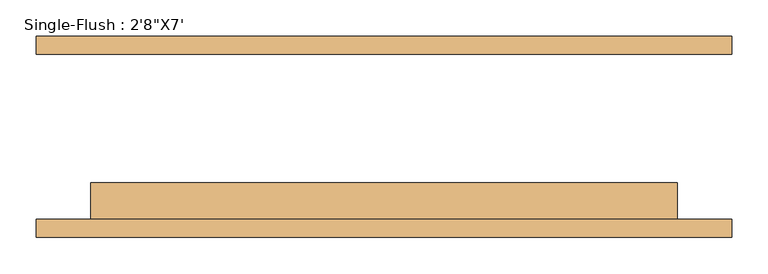
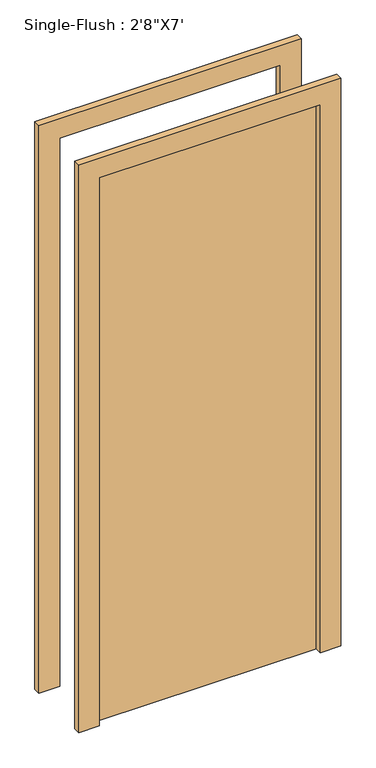
"""IFC4 building model written with IfcOpenShell, lengths in millimetres: door geometry."""

from ifc_helpers import new_model, si_unit, frame, origin, origin_with_axes, place, context, project, spatial, polyline, outline, extrude, source, transform, mapped, element, save


def door_7b345704(model_context):
    return source(origin(), model_context, "Body", "SweptSolid", [
        extrude(outline(polyline([(2209.8, -482.6), (0.0, -482.6), (0.0, -406.4), (2133.6, -406.4), (2133.6, 406.4), (0.0, 406.4), (0.0, 482.6), (2209.8, 482.6), (2209.8, -482.6)])), frame((0.0, -139.7, 0.0), z_axis=(0.0, 1.0, 0.0), x_axis=(0.0, 0.0, 1.0)), (0.0, 0.0, 1.0), 25.4),
        extrude(outline(polyline([(2209.8, 482.6), (2209.8, -482.6), (0.0, -482.6), (0.0, -406.4), (2133.6, -406.4), (2133.6, 406.4), (0.0, 406.4), (0.0, 482.6), (2209.8, 482.6)])), frame((0.0, 114.3, 0.0), z_axis=(0.0, 1.0, 0.0), x_axis=(0.0, 0.0, 1.0)), (0.0, 0.0, 1.0), 25.4),
        extrude(outline(polyline([(406.4, -63.5), (406.4, -114.3), (-406.4, -114.3), (-406.4, -63.5), (406.4, -63.5)])), origin_with_axes(), (0.0, 0.0, 1.0), 2133.6),
    ])


if __name__ == "__main__":
    model = new_model("IFC4")
    model_context = context("Model", 3, world=origin())
    ifc_project = project(units=[si_unit("LENGTHUNIT", "METRE", prefix="MILLI")], contexts=[model_context])
    site = spatial("IfcSite", under=ifc_project)
    building = spatial("IfcBuilding", under=site)
    placement = place(None, origin())
    door_shape = door_7b345704(model_context)
    element("IfcDoor", 1, ObjectType="Single-Flush : 2'8\"X7'", at=placement, inside=building, context=model_context, shape_type="MappedRepresentation", body=[
        mapped(door_shape, transform((0.0, 0.0, 0.0), x_axis=(1.0, 0.0, 0.0), y_axis=(0.0, 1.0, 0.0), z_axis=(0.0, 0.0, 1.0))),
    ])
    save(model, "model.ifc")

# Revit data of these elements
# Type "Single-Flush : 2'8\"X7'"
#   Type Mark = "12"
#   Construction Type Id = "MDOOR"
#   Assembly Code = "C1020"
#   Analytic Construction = "Metal"
#   Thickness = 0' - 2"
#   Heat Transfer Coefficient (U) = 0.651978 BTU/(h·ft²·°F)
#   Height = 7' - 0"
#   Trim Projection Ext = 0' - 1"
#   Trim Projection Int = 0' - 1"
#   Trim Width = 0' - 3"
#   Width = 2' - 8"
#   Define Thermal Properties by = 1
#   Door Material = Door - Panel
#   Frame Material = Door - Frame
#   Visual Light Transmittance = 0
#   Solar Heat Gain Coefficient = 0
#   Function = (empty or 0)
#   Wall Closure = (empty or 0)
# Element 1 (IfcDoor, "Single-Flush : 2'8\"X7'")
#   Materials on its faces: "Door - Frame", "Door - Panel"
# Materials
#   "Door - Panel": class "Wood", colour RGB 210 159 95, transparency 0, Cost = 0
#   "Door - Frame": colour RGB 118 70 51, transparency 0, Cost = 0
